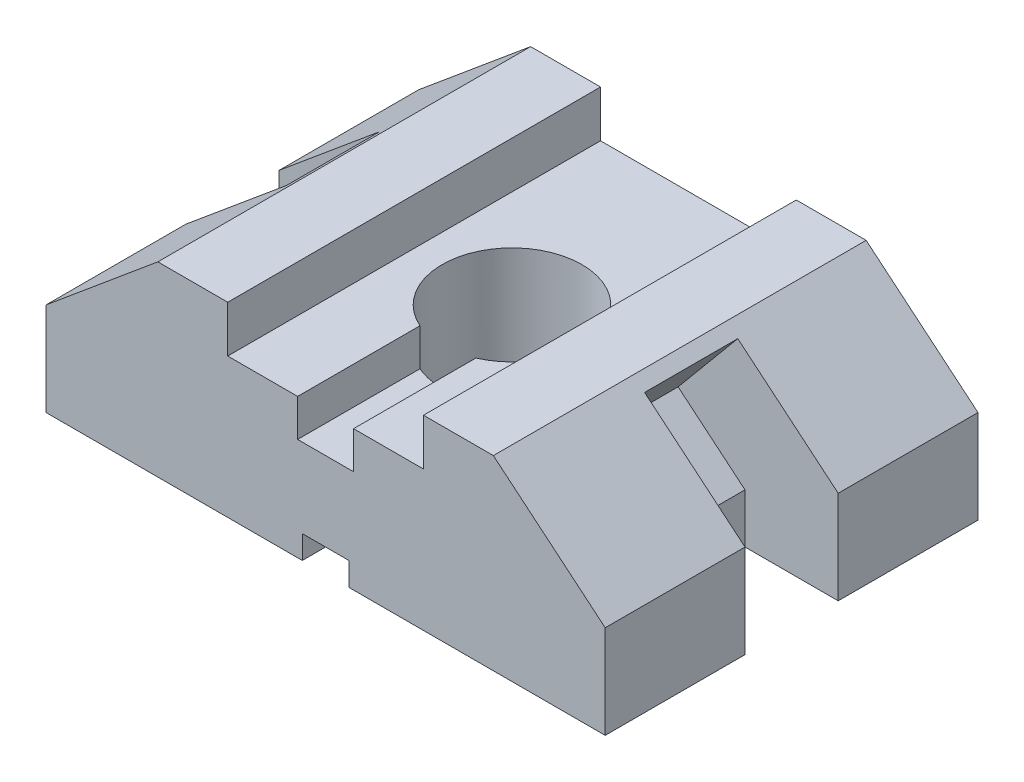
ISO-10303-21;
HEADER;
FILE_DESCRIPTION(('STEP AP214'),'2;1');
FILE_NAME('part.step','',(''),(''),'','','');
FILE_SCHEMA(('AUTOMOTIVE_DESIGN { 1 0 10303 214 1 1 1 1 }'));
ENDSEC;
DATA;
#1=APPLICATION_CONTEXT('core data for automotive mechanical design processes');
#2=APPLICATION_PROTOCOL_DEFINITION('international standard','automotive_design',2000,#1);
#3=PRODUCT_CONTEXT('',#1,'mechanical');
#4=PRODUCT('Part','Part','',(#3));
#5=PRODUCT_RELATED_PRODUCT_CATEGORY('part','',(#4));
#6=PRODUCT_DEFINITION_FORMATION('','',#4);
#7=PRODUCT_DEFINITION_CONTEXT('part definition',#1,'design');
#8=PRODUCT_DEFINITION('design','',#6,#7);
#9=PRODUCT_DEFINITION_SHAPE('','',#8);
#10=(LENGTH_UNIT() NAMED_UNIT(*) SI_UNIT(.MILLI.,.METRE.));
#11=(NAMED_UNIT(*) PLANE_ANGLE_UNIT() SI_UNIT($,.RADIAN.));
#12=(NAMED_UNIT(*) SI_UNIT($,.STERADIAN.) SOLID_ANGLE_UNIT());
#13=UNCERTAINTY_MEASURE_WITH_UNIT(LENGTH_MEASURE(1.E-05),#10,'distance_accuracy_value','');
#14=(GEOMETRIC_REPRESENTATION_CONTEXT(3) GLOBAL_UNCERTAINTY_ASSIGNED_CONTEXT((#13)) GLOBAL_UNIT_ASSIGNED_CONTEXT((#10,
#11,#12)) REPRESENTATION_CONTEXT('',''));
#15=CARTESIAN_POINT('',(0.,0.,0.));
#16=DIRECTION('',(0.,0.,1.));
#17=DIRECTION('',(1.,0.,0.));
#18=AXIS2_PLACEMENT_3D('',#15,#16,#17);
#19=CARTESIAN_POINT('',(0.,0.,80.));
#20=DIRECTION('',(1.,0.,0.));
#21=DIRECTION('',(0.,0.,-1.));
#22=AXIS2_PLACEMENT_3D('',#19,#20,#21);
#23=PLANE('',#22);
#24=DIRECTION('',(0.,0.,-1.));
#25=VECTOR('',#24,1.);
#26=CARTESIAN_POINT('',(0.,0.,80.));
#27=LINE('',#26,#25);
#28=CARTESIAN_POINT('',(0.,0.,30.));
#29=VERTEX_POINT('',#28);
#30=CARTESIAN_POINT('',(0.,0.,0.));
#31=VERTEX_POINT('',#30);
#32=EDGE_CURVE('E418',#29,#31,#27,.T.);
#33=ORIENTED_EDGE('',*,*,#32,.F.);
#34=DIRECTION('',(0.,-1.,0.));
#35=VECTOR('',#34,1.);
#36=CARTESIAN_POINT('',(0.,20.,30.));
#37=LINE('',#36,#35);
#38=CARTESIAN_POINT('',(0.,20.,30.));
#39=VERTEX_POINT('',#38);
#40=EDGE_CURVE('E286',#39,#29,#37,.T.);
#41=ORIENTED_EDGE('',*,*,#40,.F.);
#42=DIRECTION('',(0.,0.,-1.));
#43=VECTOR('',#42,1.);
#44=CARTESIAN_POINT('',(0.,20.,80.));
#45=LINE('',#44,#43);
#46=CARTESIAN_POINT('',(0.,20.,0.));
#47=VERTEX_POINT('',#46);
#48=EDGE_CURVE('E460',#39,#47,#45,.T.);
#49=ORIENTED_EDGE('',*,*,#48,.T.);
#50=DIRECTION('',(0.,-1.,0.));
#51=VECTOR('',#50,1.);
#52=CARTESIAN_POINT('',(0.,0.,0.));
#53=LINE('',#52,#51);
#54=EDGE_CURVE('E388',#47,#31,#53,.T.);
#55=ORIENTED_EDGE('',*,*,#54,.T.);
#56=EDGE_LOOP('',(#33,#41,#49,#55));
#57=FACE_BOUND('',#56,.T.);
#58=ADVANCED_FACE('F44',(#57),#23,.F.);
#59=CARTESIAN_POINT('',(120.,0.,80.));
#60=DIRECTION('',(-1.,0.,0.));
#61=DIRECTION('',(0.,0.,1.));
#62=AXIS2_PLACEMENT_3D('',#59,#60,#61);
#63=PLANE('',#62);
#64=DIRECTION('',(0.,0.,-1.));
#65=VECTOR('',#64,1.);
#66=CARTESIAN_POINT('',(120.,0.,80.));
#67=LINE('',#66,#65);
#68=CARTESIAN_POINT('',(120.,0.,80.));
#69=VERTEX_POINT('',#68);
#70=CARTESIAN_POINT('',(120.,0.,50.));
#71=VERTEX_POINT('',#70);
#72=EDGE_CURVE('E484',#69,#71,#67,.T.);
#73=ORIENTED_EDGE('',*,*,#72,.T.);
#74=DIRECTION('',(0.,-1.,0.));
#75=VECTOR('',#74,1.);
#76=CARTESIAN_POINT('',(120.,20.,50.));
#77=LINE('',#76,#75);
#78=CARTESIAN_POINT('',(120.,20.,50.));
#79=VERTEX_POINT('',#78);
#80=EDGE_CURVE('E321',#79,#71,#77,.T.);
#81=ORIENTED_EDGE('',*,*,#80,.F.);
#82=DIRECTION('',(0.,0.,-1.));
#83=VECTOR('',#82,1.);
#84=CARTESIAN_POINT('',(120.,20.,80.));
#85=LINE('',#84,#83);
#86=CARTESIAN_POINT('',(120.,20.,80.));
#87=VERTEX_POINT('',#86);
#88=EDGE_CURVE('E478',#87,#79,#85,.T.);
#89=ORIENTED_EDGE('',*,*,#88,.F.);
#90=DIRECTION('',(0.,1.,0.));
#91=VECTOR('',#90,1.);
#92=CARTESIAN_POINT('',(120.,0.,80.));
#93=LINE('',#92,#91);
#94=EDGE_CURVE('E398',#69,#87,#93,.T.);
#95=ORIENTED_EDGE('',*,*,#94,.F.);
#96=EDGE_LOOP('',(#73,#81,#89,#95));
#97=FACE_BOUND('',#96,.T.);
#98=ADVANCED_FACE('F549',(#97),#63,.F.);
#99=CARTESIAN_POINT('',(55.,0.,80.));
#100=DIRECTION('',(-1.,0.,0.));
#101=DIRECTION('',(0.,0.,1.));
#102=AXIS2_PLACEMENT_3D('',#99,#100,#101);
#103=PLANE('',#102);
#104=DIRECTION('',(0.,0.,-1.));
#105=VECTOR('',#104,1.);
#106=CARTESIAN_POINT('',(55.,0.,80.));
#107=LINE('',#106,#105);
#108=CARTESIAN_POINT('',(55.,0.,80.));
#109=VERTEX_POINT('',#108);
#110=CARTESIAN_POINT('',(55.,0.,54.142135623731));
#111=VERTEX_POINT('',#110);
#112=EDGE_CURVE('E499',#109,#111,#107,.T.);
#113=ORIENTED_EDGE('',*,*,#112,.T.);
#114=DIRECTION('',(0.,1.,0.));
#115=VECTOR('',#114,1.);
#116=CARTESIAN_POINT('',(55.,-50.,54.142135623731));
#117=LINE('',#116,#115);
#118=CARTESIAN_POINT('',(55.,5.,54.142135623731));
#119=VERTEX_POINT('',#118);
#120=EDGE_CURVE('E378',#111,#119,#117,.T.);
#121=ORIENTED_EDGE('',*,*,#120,.T.);
#122=DIRECTION('',(0.,0.,-1.));
#123=VECTOR('',#122,1.);
#124=CARTESIAN_POINT('',(55.,5.,80.));
#125=LINE('',#124,#123);
#126=CARTESIAN_POINT('',(55.,5.,80.));
#127=VERTEX_POINT('',#126);
#128=EDGE_CURVE('E496',#127,#119,#125,.T.);
#129=ORIENTED_EDGE('',*,*,#128,.F.);
#130=DIRECTION('',(0.,1.,0.));
#131=VECTOR('',#130,1.);
#132=CARTESIAN_POINT('',(55.,0.,80.));
#133=LINE('',#132,#131);
#134=EDGE_CURVE('E386',#109,#127,#133,.T.);
#135=ORIENTED_EDGE('',*,*,#134,.F.);
#136=EDGE_LOOP('',(#113,#121,#129,#135));
#137=FACE_BOUND('',#136,.T.);
#138=ADVANCED_FACE('F568',(#137),#103,.F.);
#139=CARTESIAN_POINT('',(55.,5.,80.));
#140=DIRECTION('',(0.,1.,0.));
#141=DIRECTION('',(0.,0.,1.));
#142=AXIS2_PLACEMENT_3D('',#139,#140,#141);
#143=PLANE('',#142);
#144=DIRECTION('',(0.,0.,-1.));
#145=VECTOR('',#144,1.);
#146=CARTESIAN_POINT('',(65.,5.,80.));
#147=LINE('',#146,#145);
#148=CARTESIAN_POINT('',(65.,5.,25.857864376269));
#149=VERTEX_POINT('',#148);
#150=CARTESIAN_POINT('',(65.,5.,0.));
#151=VERTEX_POINT('',#150);
#152=EDGE_CURVE('E493',#149,#151,#147,.T.);
#153=ORIENTED_EDGE('',*,*,#152,.F.);
#154=CARTESIAN_POINT('',(60.,5.,40.));
#155=DIRECTION('',(0.,1.,0.));
#156=DIRECTION('',(0.,0.,1.));
#157=AXIS2_PLACEMENT_3D('',#154,#155,#156);
#158=CIRCLE('',#157,15.);
#159=CARTESIAN_POINT('',(55.,5.,25.8578643762691));
#160=VERTEX_POINT('',#159);
#161=EDGE_CURVE('E374',#149,#160,#158,.T.);
#162=ORIENTED_EDGE('',*,*,#161,.T.);
#163=CARTESIAN_POINT('',(55.,5.,0.));
#164=VERTEX_POINT('',#163);
#165=EDGE_CURVE('E492',#160,#164,#125,.T.);
#166=ORIENTED_EDGE('',*,*,#165,.T.);
#167=DIRECTION('',(1.,0.,0.));
#168=VECTOR('',#167,1.);
#169=CARTESIAN_POINT('',(55.,5.,0.));
#170=LINE('',#169,#168);
#171=EDGE_CURVE('E425',#164,#151,#170,.T.);
#172=ORIENTED_EDGE('',*,*,#171,.T.);
#173=EDGE_LOOP('',(#153,#162,#166,#172));
#174=FACE_BOUND('',#173,.T.);
#175=ADVANCED_FACE('F590',(#174),#143,.F.);
#176=CARTESIAN_POINT('',(65.,5.,80.));
#177=DIRECTION('',(1.,0.,0.));
#178=DIRECTION('',(0.,0.,-1.));
#179=AXIS2_PLACEMENT_3D('',#176,#177,#178);
#180=PLANE('',#179);
#181=DIRECTION('',(0.,0.,-1.));
#182=VECTOR('',#181,1.);
#183=CARTESIAN_POINT('',(65.,0.,80.));
#184=LINE('',#183,#182);
#185=CARTESIAN_POINT('',(65.,0.,25.857864376269));
#186=VERTEX_POINT('',#185);
#187=CARTESIAN_POINT('',(65.,0.,0.));
#188=VERTEX_POINT('',#187);
#189=EDGE_CURVE('E487',#186,#188,#184,.T.);
#190=ORIENTED_EDGE('',*,*,#189,.F.);
#191=DIRECTION('',(0.,1.,0.));
#192=VECTOR('',#191,1.);
#193=CARTESIAN_POINT('',(65.,-50.,25.857864376269));
#194=LINE('',#193,#192);
#195=EDGE_CURVE('E367',#186,#149,#194,.T.);
#196=ORIENTED_EDGE('',*,*,#195,.T.);
#197=ORIENTED_EDGE('',*,*,#152,.T.);
#198=DIRECTION('',(0.,-1.,0.));
#199=VECTOR('',#198,1.);
#200=CARTESIAN_POINT('',(65.,5.,0.));
#201=LINE('',#200,#199);
#202=EDGE_CURVE('E430',#151,#188,#201,.T.);
#203=ORIENTED_EDGE('',*,*,#202,.T.);
#204=EDGE_LOOP('',(#190,#196,#197,#203));
#205=FACE_BOUND('',#204,.T.);
#206=ADVANCED_FACE('F588',(#205),#180,.F.);
#207=CARTESIAN_POINT('',(0.,0.,80.));
#208=DIRECTION('',(0.,1.,0.));
#209=DIRECTION('',(0.,0.,1.));
#210=AXIS2_PLACEMENT_3D('',#207,#208,#209);
#211=PLANE('',#210);
#212=DIRECTION('',(0.,0.,1.));
#213=VECTOR('',#212,1.);
#214=CARTESIAN_POINT('',(20.,0.,30.));
#215=LINE('',#214,#213);
#216=CARTESIAN_POINT('',(20.,0.,30.));
#217=VERTEX_POINT('',#216);
#218=CARTESIAN_POINT('',(20.,0.,50.));
#219=VERTEX_POINT('',#218);
#220=EDGE_CURVE('E295',#217,#219,#215,.T.);
#221=ORIENTED_EDGE('',*,*,#220,.F.);
#222=DIRECTION('',(-1.,0.,0.));
#223=VECTOR('',#222,1.);
#224=CARTESIAN_POINT('',(20.,0.,30.));
#225=LINE('',#224,#223);
#226=EDGE_CURVE('E297',#217,#29,#225,.T.);
#227=ORIENTED_EDGE('',*,*,#226,.T.);
#228=ORIENTED_EDGE('',*,*,#32,.T.);
#229=DIRECTION('',(1.,0.,0.));
#230=VECTOR('',#229,1.);
#231=CARTESIAN_POINT('',(0.,0.,0.));
#232=LINE('',#231,#230);
#233=CARTESIAN_POINT('',(55.,0.,0.));
#234=VERTEX_POINT('',#233);
#235=EDGE_CURVE('E383',#31,#234,#232,.T.);
#236=ORIENTED_EDGE('',*,*,#235,.T.);
#237=CARTESIAN_POINT('',(55.,0.,25.8578643762691));
#238=VERTEX_POINT('',#237);
#239=EDGE_CURVE('E497',#238,#234,#107,.T.);
#240=ORIENTED_EDGE('',*,*,#239,.F.);
#241=CARTESIAN_POINT('',(60.,0.,40.));
#242=DIRECTION('',(0.,1.,0.));
#243=DIRECTION('',(0.,0.,1.));
#244=AXIS2_PLACEMENT_3D('',#241,#242,#243);
#245=CIRCLE('',#244,15.);
#246=EDGE_CURVE('E385',#238,#111,#245,.T.);
#247=ORIENTED_EDGE('',*,*,#246,.T.);
#248=ORIENTED_EDGE('',*,*,#112,.F.);
#249=DIRECTION('',(1.,0.,0.));
#250=VECTOR('',#249,1.);
#251=CARTESIAN_POINT('',(0.,0.,80.));
#252=LINE('',#251,#250);
#253=CARTESIAN_POINT('',(0.,0.,80.));
#254=VERTEX_POINT('',#253);
#255=EDGE_CURVE('E387',#254,#109,#252,.T.);
#256=ORIENTED_EDGE('',*,*,#255,.F.);
#257=CARTESIAN_POINT('',(0.,0.,50.));
#258=VERTEX_POINT('',#257);
#259=EDGE_CURVE('E451',#254,#258,#27,.T.);
#260=ORIENTED_EDGE('',*,*,#259,.T.);
#261=DIRECTION('',(-1.,0.,0.));
#262=VECTOR('',#261,1.);
#263=CARTESIAN_POINT('',(20.,0.,50.));
#264=LINE('',#263,#262);
#265=EDGE_CURVE('E70',#219,#258,#264,.T.);
#266=ORIENTED_EDGE('',*,*,#265,.F.);
#267=EDGE_LOOP('',(#221,#227,#228,#236,#240,#247,#248,#256,#260,#266));
#268=FACE_BOUND('',#267,.T.);
#269=ADVANCED_FACE('F50',(#268),#211,.F.);
#270=ORIENTED_EDGE('',*,*,#165,.F.);
#271=DIRECTION('',(0.,1.,0.));
#272=VECTOR('',#271,1.);
#273=CARTESIAN_POINT('',(55.,-50.,25.8578643762691));
#274=LINE('',#273,#272);
#275=EDGE_CURVE('E376',#160,#238,#274,.F.);
#276=ORIENTED_EDGE('',*,*,#275,.T.);
#277=ORIENTED_EDGE('',*,*,#239,.T.);
#278=DIRECTION('',(0.,1.,0.));
#279=VECTOR('',#278,1.);
#280=CARTESIAN_POINT('',(55.,0.,0.));
#281=LINE('',#280,#279);
#282=EDGE_CURVE('E423',#234,#164,#281,.T.);
#283=ORIENTED_EDGE('',*,*,#282,.T.);
#284=EDGE_LOOP('',(#270,#276,#277,#283));
#285=FACE_BOUND('',#284,.T.);
#286=ADVANCED_FACE('F579',(#285),#103,.F.);
#287=ORIENTED_EDGE('',*,*,#128,.T.);
#288=CARTESIAN_POINT('',(65.,5.,54.142135623731));
#289=VERTEX_POINT('',#288);
#290=EDGE_CURVE('E375',#119,#289,#158,.T.);
#291=ORIENTED_EDGE('',*,*,#290,.T.);
#292=CARTESIAN_POINT('',(65.,5.,80.));
#293=VERTEX_POINT('',#292);
#294=EDGE_CURVE('E495',#293,#289,#147,.T.);
#295=ORIENTED_EDGE('',*,*,#294,.F.);
#296=DIRECTION('',(1.,0.,0.));
#297=VECTOR('',#296,1.);
#298=CARTESIAN_POINT('',(55.,5.,80.));
#299=LINE('',#298,#297);
#300=EDGE_CURVE('E395',#127,#293,#299,.T.);
#301=ORIENTED_EDGE('',*,*,#300,.F.);
#302=EDGE_LOOP('',(#287,#291,#295,#301));
#303=FACE_BOUND('',#302,.T.);
#304=ADVANCED_FACE('F562',(#303),#143,.F.);
#305=ORIENTED_EDGE('',*,*,#294,.T.);
#306=DIRECTION('',(0.,1.,0.));
#307=VECTOR('',#306,1.);
#308=CARTESIAN_POINT('',(65.,-50.,54.142135623731));
#309=LINE('',#308,#307);
#310=CARTESIAN_POINT('',(65.,0.,54.142135623731));
#311=VERTEX_POINT('',#310);
#312=EDGE_CURVE('E366',#289,#311,#309,.F.);
#313=ORIENTED_EDGE('',*,*,#312,.T.);
#314=CARTESIAN_POINT('',(65.,0.,80.));
#315=VERTEX_POINT('',#314);
#316=EDGE_CURVE('E486',#315,#311,#184,.T.);
#317=ORIENTED_EDGE('',*,*,#316,.F.);
#318=DIRECTION('',(0.,-1.,0.));
#319=VECTOR('',#318,1.);
#320=CARTESIAN_POINT('',(65.,5.,80.));
#321=LINE('',#320,#319);
#322=EDGE_CURVE('E391',#293,#315,#321,.T.);
#323=ORIENTED_EDGE('',*,*,#322,.F.);
#324=EDGE_LOOP('',(#305,#313,#317,#323));
#325=FACE_BOUND('',#324,.T.);
#326=ADVANCED_FACE('F559',(#325),#180,.F.);
#327=CARTESIAN_POINT('',(65.,0.,80.));
#328=DIRECTION('',(0.,1.,0.));
#329=DIRECTION('',(0.,0.,1.));
#330=AXIS2_PLACEMENT_3D('',#327,#328,#329);
#331=PLANE('',#330);
#332=DIRECTION('',(0.,0.,-1.));
#333=VECTOR('',#332,1.);
#334=CARTESIAN_POINT('',(100.,0.,50.));
#335=LINE('',#334,#333);
#336=CARTESIAN_POINT('',(100.,0.,50.));
#337=VERTEX_POINT('',#336);
#338=CARTESIAN_POINT('',(100.,0.,30.));
#339=VERTEX_POINT('',#338);
#340=EDGE_CURVE('E329',#337,#339,#335,.T.);
#341=ORIENTED_EDGE('',*,*,#340,.F.);
#342=DIRECTION('',(1.,0.,0.));
#343=VECTOR('',#342,1.);
#344=CARTESIAN_POINT('',(100.,0.,50.));
#345=LINE('',#344,#343);
#346=EDGE_CURVE('E331',#337,#71,#345,.T.);
#347=ORIENTED_EDGE('',*,*,#346,.T.);
#348=ORIENTED_EDGE('',*,*,#72,.F.);
#349=DIRECTION('',(1.,0.,0.));
#350=VECTOR('',#349,1.);
#351=CARTESIAN_POINT('',(65.,0.,80.));
#352=LINE('',#351,#350);
#353=EDGE_CURVE('E397',#315,#69,#352,.T.);
#354=ORIENTED_EDGE('',*,*,#353,.F.);
#355=ORIENTED_EDGE('',*,*,#316,.T.);
#356=CARTESIAN_POINT('',(60.,0.,40.));
#357=DIRECTION('',(0.,1.,0.));
#358=DIRECTION('',(0.,0.,1.));
#359=AXIS2_PLACEMENT_3D('',#356,#357,#358);
#360=CIRCLE('',#359,15.);
#361=EDGE_CURVE('E361',#311,#186,#360,.T.);
#362=ORIENTED_EDGE('',*,*,#361,.T.);
#363=ORIENTED_EDGE('',*,*,#189,.T.);
#364=DIRECTION('',(1.,0.,0.));
#365=VECTOR('',#364,1.);
#366=CARTESIAN_POINT('',(65.,0.,0.));
#367=LINE('',#366,#365);
#368=CARTESIAN_POINT('',(120.,0.,0.));
#369=VERTEX_POINT('',#368);
#370=EDGE_CURVE('E427',#188,#369,#367,.T.);
#371=ORIENTED_EDGE('',*,*,#370,.T.);
#372=CARTESIAN_POINT('',(120.,0.,30.));
#373=VERTEX_POINT('',#372);
#374=EDGE_CURVE('E483',#373,#369,#67,.T.);
#375=ORIENTED_EDGE('',*,*,#374,.F.);
#376=DIRECTION('',(1.,0.,0.));
#377=VECTOR('',#376,1.);
#378=CARTESIAN_POINT('',(100.,0.,30.));
#379=LINE('',#378,#377);
#380=EDGE_CURVE('E339',#339,#373,#379,.T.);
#381=ORIENTED_EDGE('',*,*,#380,.F.);
#382=EDGE_LOOP('',(#341,#347,#348,#354,#355,#362,#363,#371,#375,#381));
#383=FACE_BOUND('',#382,.T.);
#384=ADVANCED_FACE('F528',(#383),#331,.F.);
#385=CARTESIAN_POINT('',(120.,20.,30.));
#386=VERTEX_POINT('',#385);
#387=CARTESIAN_POINT('',(120.,20.,0.));
#388=VERTEX_POINT('',#387);
#389=EDGE_CURVE('E476',#386,#388,#85,.T.);
#390=ORIENTED_EDGE('',*,*,#389,.F.);
#391=DIRECTION('',(0.,1.,0.));
#392=VECTOR('',#391,1.);
#393=CARTESIAN_POINT('',(120.,20.,30.));
#394=LINE('',#393,#392);
#395=EDGE_CURVE('E326',#373,#386,#394,.T.);
#396=ORIENTED_EDGE('',*,*,#395,.F.);
#397=ORIENTED_EDGE('',*,*,#374,.T.);
#398=DIRECTION('',(0.,1.,0.));
#399=VECTOR('',#398,1.);
#400=CARTESIAN_POINT('',(120.,0.,0.));
#401=LINE('',#400,#399);
#402=EDGE_CURVE('E433',#369,#388,#401,.T.);
#403=ORIENTED_EDGE('',*,*,#402,.T.);
#404=EDGE_LOOP('',(#390,#396,#397,#403));
#405=FACE_BOUND('',#404,.T.);
#406=ADVANCED_FACE('F535',(#405),#63,.F.);
#407=CARTESIAN_POINT('',(96.,40.,80.));
#408=DIRECTION('',(-0.64018439966448,-0.768221279597376,0.));
#409=DIRECTION('',(0.768221279597376,-0.64018439966448,0.));
#410=AXIS2_PLACEMENT_3D('',#407,#408,#409);
#411=PLANE('',#410);
#412=DIRECTION('',(0.,0.,1.));
#413=VECTOR('',#412,1.);
#414=CARTESIAN_POINT('',(98.4512258008987,37.9573118325844,50.));
#415=LINE('',#414,#413);
#416=CARTESIAN_POINT('',(98.4512258008987,37.9573118325844,30.));
#417=VERTEX_POINT('',#416);
#418=CARTESIAN_POINT('',(98.4512258008987,37.9573118325844,50.));
#419=VERTEX_POINT('',#418);
#420=EDGE_CURVE('E319',#417,#419,#415,.T.);
#421=ORIENTED_EDGE('',*,*,#420,.F.);
#422=DIRECTION('',(-0.768221279597376,0.64018439966448,0.));
#423=VECTOR('',#422,1.);
#424=CARTESIAN_POINT('',(98.4512258008987,37.9573118325844,30.));
#425=LINE('',#424,#423);
#426=EDGE_CURVE('E302',#386,#417,#425,.T.);
#427=ORIENTED_EDGE('',*,*,#426,.F.);
#428=ORIENTED_EDGE('',*,*,#389,.T.);
#429=DIRECTION('',(-0.768221279597376,0.64018439966448,0.));
#430=VECTOR('',#429,1.);
#431=CARTESIAN_POINT('',(96.,40.,0.));
#432=LINE('',#431,#430);
#433=CARTESIAN_POINT('',(96.,40.,0.));
#434=VERTEX_POINT('',#433);
#435=EDGE_CURVE('E436',#388,#434,#432,.T.);
#436=ORIENTED_EDGE('',*,*,#435,.T.);
#437=DIRECTION('',(0.,0.,-1.));
#438=VECTOR('',#437,1.);
#439=CARTESIAN_POINT('',(96.,40.,80.));
#440=LINE('',#439,#438);
#441=CARTESIAN_POINT('',(96.,40.,80.));
#442=VERTEX_POINT('',#441);
#443=EDGE_CURVE('E477',#442,#434,#440,.T.);
#444=ORIENTED_EDGE('',*,*,#443,.F.);
#445=DIRECTION('',(-0.768221279597376,0.64018439966448,0.));
#446=VECTOR('',#445,1.);
#447=CARTESIAN_POINT('',(96.,40.,80.));
#448=LINE('',#447,#446);
#449=EDGE_CURVE('E396',#87,#442,#448,.T.);
#450=ORIENTED_EDGE('',*,*,#449,.F.);
#451=ORIENTED_EDGE('',*,*,#88,.T.);
#452=DIRECTION('',(0.768221279597376,-0.64018439966448,0.));
#453=VECTOR('',#452,1.);
#454=CARTESIAN_POINT('',(120.,20.,50.));
#455=LINE('',#454,#453);
#456=EDGE_CURVE('E309',#419,#79,#455,.T.);
#457=ORIENTED_EDGE('',*,*,#456,.F.);
#458=EDGE_LOOP('',(#421,#427,#428,#436,#444,#450,#451,#457));
#459=FACE_BOUND('',#458,.T.);
#460=ADVANCED_FACE('F540',(#459),#411,.F.);
#461=CARTESIAN_POINT('',(81.,40.,80.));
#462=DIRECTION('',(0.,-1.,0.));
#463=DIRECTION('',(0.,0.,-1.));
#464=AXIS2_PLACEMENT_3D('',#461,#462,#463);
#465=PLANE('',#464);
#466=DIRECTION('',(-1.,0.,0.));
#467=VECTOR('',#466,1.);
#468=CARTESIAN_POINT('',(81.,40.,0.));
#469=LINE('',#468,#467);
#470=CARTESIAN_POINT('',(81.,40.,0.));
#471=VERTEX_POINT('',#470);
#472=EDGE_CURVE('E438',#434,#471,#469,.T.);
#473=ORIENTED_EDGE('',*,*,#472,.T.);
#474=DIRECTION('',(0.,0.,-1.));
#475=VECTOR('',#474,1.);
#476=CARTESIAN_POINT('',(81.,40.,80.));
#477=LINE('',#476,#475);
#478=CARTESIAN_POINT('',(81.,40.,80.));
#479=VERTEX_POINT('',#478);
#480=EDGE_CURVE('E474',#479,#471,#477,.T.);
#481=ORIENTED_EDGE('',*,*,#480,.F.);
#482=DIRECTION('',(-1.,0.,0.));
#483=VECTOR('',#482,1.);
#484=CARTESIAN_POINT('',(81.,40.,80.));
#485=LINE('',#484,#483);
#486=EDGE_CURVE('E405',#442,#479,#485,.T.);
#487=ORIENTED_EDGE('',*,*,#486,.F.);
#488=ORIENTED_EDGE('',*,*,#443,.T.);
#489=EDGE_LOOP('',(#473,#481,#487,#488));
#490=FACE_BOUND('',#489,.T.);
#491=ADVANCED_FACE('F591',(#490),#465,.F.);
#492=CARTESIAN_POINT('',(81.,30.,80.));
#493=DIRECTION('',(1.,0.,0.));
#494=DIRECTION('',(0.,0.,-1.));
#495=AXIS2_PLACEMENT_3D('',#492,#493,#494);
#496=PLANE('',#495);
#497=DIRECTION('',(0.,-1.,0.));
#498=VECTOR('',#497,1.);
#499=CARTESIAN_POINT('',(81.,30.,0.));
#500=LINE('',#499,#498);
#501=CARTESIAN_POINT('',(81.,30.,0.));
#502=VERTEX_POINT('',#501);
#503=EDGE_CURVE('E439',#471,#502,#500,.T.);
#504=ORIENTED_EDGE('',*,*,#503,.T.);
#505=DIRECTION('',(0.,0.,-1.));
#506=VECTOR('',#505,1.);
#507=CARTESIAN_POINT('',(81.,30.,80.));
#508=LINE('',#507,#506);
#509=CARTESIAN_POINT('',(81.,30.,80.));
#510=VERTEX_POINT('',#509);
#511=EDGE_CURVE('E468',#510,#502,#508,.T.);
#512=ORIENTED_EDGE('',*,*,#511,.F.);
#513=DIRECTION('',(0.,-1.,0.));
#514=VECTOR('',#513,1.);
#515=CARTESIAN_POINT('',(81.,30.,80.));
#516=LINE('',#515,#514);
#517=EDGE_CURVE('E404',#479,#510,#516,.T.);
#518=ORIENTED_EDGE('',*,*,#517,.F.);
#519=ORIENTED_EDGE('',*,*,#480,.T.);
#520=EDGE_LOOP('',(#504,#512,#518,#519));
#521=FACE_BOUND('',#520,.T.);
#522=ADVANCED_FACE('F599',(#521),#496,.F.);
#523=CARTESIAN_POINT('',(54.,30.,80.));
#524=DIRECTION('',(0.,-1.,0.));
#525=DIRECTION('',(0.,0.,-1.));
#526=AXIS2_PLACEMENT_3D('',#523,#524,#525);
#527=PLANE('',#526);
#528=CARTESIAN_POINT('',(60.,30.,40.));
#529=DIRECTION('',(0.,1.,0.));
#530=DIRECTION('',(0.,0.,1.));
#531=AXIS2_PLACEMENT_3D('',#528,#529,#530);
#532=CIRCLE('',#531,15.);
#533=CARTESIAN_POINT('',(66.,30.,53.7477270848675));
#534=VERTEX_POINT('',#533);
#535=CARTESIAN_POINT('',(54.,30.,53.7477270848675));
#536=VERTEX_POINT('',#535);
#537=EDGE_CURVE('E351',#534,#536,#532,.T.);
#538=ORIENTED_EDGE('',*,*,#537,.F.);
#539=DIRECTION('',(0.,0.,1.));
#540=VECTOR('',#539,1.);
#541=CARTESIAN_POINT('',(66.,30.,50.));
#542=LINE('',#541,#540);
#543=CARTESIAN_POINT('',(66.,30.,80.));
#544=VERTEX_POINT('',#543);
#545=EDGE_CURVE('E355',#534,#544,#542,.T.);
#546=ORIENTED_EDGE('',*,*,#545,.T.);
#547=DIRECTION('',(-1.,0.,0.));
#548=VECTOR('',#547,1.);
#549=CARTESIAN_POINT('',(66.,30.,80.));
#550=LINE('',#549,#548);
#551=EDGE_CURVE('E410',#510,#544,#550,.T.);
#552=ORIENTED_EDGE('',*,*,#551,.F.);
#553=ORIENTED_EDGE('',*,*,#511,.T.);
#554=DIRECTION('',(-1.,0.,0.));
#555=VECTOR('',#554,1.);
#556=CARTESIAN_POINT('',(54.,30.,0.));
#557=LINE('',#556,#555);
#558=CARTESIAN_POINT('',(39.,30.,0.));
#559=VERTEX_POINT('',#558);
#560=EDGE_CURVE('E442',#502,#559,#557,.T.);
#561=ORIENTED_EDGE('',*,*,#560,.T.);
#562=DIRECTION('',(0.,0.,-1.));
#563=VECTOR('',#562,1.);
#564=CARTESIAN_POINT('',(39.,30.,80.));
#565=LINE('',#564,#563);
#566=CARTESIAN_POINT('',(39.,30.,80.));
#567=VERTEX_POINT('',#566);
#568=EDGE_CURVE('E470',#567,#559,#565,.T.);
#569=ORIENTED_EDGE('',*,*,#568,.F.);
#570=CARTESIAN_POINT('',(54.,30.,80.));
#571=VERTEX_POINT('',#570);
#572=EDGE_CURVE('E407',#571,#567,#550,.T.);
#573=ORIENTED_EDGE('',*,*,#572,.F.);
#574=DIRECTION('',(0.,0.,1.));
#575=VECTOR('',#574,1.);
#576=CARTESIAN_POINT('',(54.,30.,50.));
#577=LINE('',#576,#575);
#578=EDGE_CURVE('E352',#536,#571,#577,.T.);
#579=ORIENTED_EDGE('',*,*,#578,.F.);
#580=EDGE_LOOP('',(#538,#546,#552,#553,#561,#569,#573,#579));
#581=FACE_BOUND('',#580,.T.);
#582=ADVANCED_FACE('F603',(#581),#527,.F.);
#583=CARTESIAN_POINT('',(39.,30.,80.));
#584=DIRECTION('',(-1.,0.,0.));
#585=DIRECTION('',(0.,0.,1.));
#586=AXIS2_PLACEMENT_3D('',#583,#584,#585);
#587=PLANE('',#586);
#588=DIRECTION('',(0.,1.,0.));
#589=VECTOR('',#588,1.);
#590=CARTESIAN_POINT('',(39.,30.,0.));
#591=LINE('',#590,#589);
#592=CARTESIAN_POINT('',(39.,40.,0.));
#593=VERTEX_POINT('',#592);
#594=EDGE_CURVE('E444',#559,#593,#591,.T.);
#595=ORIENTED_EDGE('',*,*,#594,.T.);
#596=DIRECTION('',(0.,0.,-1.));
#597=VECTOR('',#596,1.);
#598=CARTESIAN_POINT('',(39.,40.,80.));
#599=LINE('',#598,#597);
#600=CARTESIAN_POINT('',(39.,40.,80.));
#601=VERTEX_POINT('',#600);
#602=EDGE_CURVE('E464',#601,#593,#599,.T.);
#603=ORIENTED_EDGE('',*,*,#602,.F.);
#604=DIRECTION('',(0.,1.,0.));
#605=VECTOR('',#604,1.);
#606=CARTESIAN_POINT('',(39.,30.,80.));
#607=LINE('',#606,#605);
#608=EDGE_CURVE('E408',#567,#601,#607,.T.);
#609=ORIENTED_EDGE('',*,*,#608,.F.);
#610=ORIENTED_EDGE('',*,*,#568,.T.);
#611=EDGE_LOOP('',(#595,#603,#609,#610));
#612=FACE_BOUND('',#611,.T.);
#613=ADVANCED_FACE('F625',(#612),#587,.F.);
#614=CARTESIAN_POINT('',(39.,40.,80.));
#615=DIRECTION('',(0.,-1.,0.));
#616=DIRECTION('',(0.,0.,-1.));
#617=AXIS2_PLACEMENT_3D('',#614,#615,#616);
#618=PLANE('',#617);
#619=DIRECTION('',(-1.,0.,0.));
#620=VECTOR('',#619,1.);
#621=CARTESIAN_POINT('',(39.,40.,0.));
#622=LINE('',#621,#620);
#623=CARTESIAN_POINT('',(24.,40.,0.));
#624=VERTEX_POINT('',#623);
#625=EDGE_CURVE('E450',#593,#624,#622,.T.);
#626=ORIENTED_EDGE('',*,*,#625,.T.);
#627=DIRECTION('',(0.,0.,-1.));
#628=VECTOR('',#627,1.);
#629=CARTESIAN_POINT('',(24.,40.,80.));
#630=LINE('',#629,#628);
#631=CARTESIAN_POINT('',(24.,40.,80.));
#632=VERTEX_POINT('',#631);
#633=EDGE_CURVE('E462',#632,#624,#630,.T.);
#634=ORIENTED_EDGE('',*,*,#633,.F.);
#635=DIRECTION('',(-1.,0.,0.));
#636=VECTOR('',#635,1.);
#637=CARTESIAN_POINT('',(39.,40.,80.));
#638=LINE('',#637,#636);
#639=EDGE_CURVE('E415',#601,#632,#638,.T.);
#640=ORIENTED_EDGE('',*,*,#639,.F.);
#641=ORIENTED_EDGE('',*,*,#602,.T.);
#642=EDGE_LOOP('',(#626,#634,#640,#641));
#643=FACE_BOUND('',#642,.T.);
#644=ADVANCED_FACE('F628',(#643),#618,.F.);
#645=CARTESIAN_POINT('',(24.,40.,80.));
#646=DIRECTION('',(0.64018439966448,-0.768221279597376,0.));
#647=DIRECTION('',(0.768221279597376,0.64018439966448,0.));
#648=AXIS2_PLACEMENT_3D('',#645,#646,#647);
#649=PLANE('',#648);
#650=ORIENTED_EDGE('',*,*,#48,.F.);
#651=DIRECTION('',(-0.768221279597376,-0.64018439966448,0.));
#652=VECTOR('',#651,1.);
#653=CARTESIAN_POINT('',(0.,20.,30.));
#654=LINE('',#653,#652);
#655=CARTESIAN_POINT('',(21.6499498332045,38.0416248610038,30.));
#656=VERTEX_POINT('',#655);
#657=EDGE_CURVE('E272',#656,#39,#654,.T.);
#658=ORIENTED_EDGE('',*,*,#657,.F.);
#659=DIRECTION('',(0.,0.,-1.));
#660=VECTOR('',#659,1.);
#661=CARTESIAN_POINT('',(21.6499498332045,38.0416248610038,30.));
#662=LINE('',#661,#660);
#663=CARTESIAN_POINT('',(21.6499498332045,38.0416248610038,50.));
#664=VERTEX_POINT('',#663);
#665=EDGE_CURVE('E290',#664,#656,#662,.T.);
#666=ORIENTED_EDGE('',*,*,#665,.F.);
#667=DIRECTION('',(0.768221279597376,0.64018439966448,0.));
#668=VECTOR('',#667,1.);
#669=CARTESIAN_POINT('',(21.6499498332045,38.0416248610038,50.));
#670=LINE('',#669,#668);
#671=CARTESIAN_POINT('',(0.,20.,50.));
#672=VERTEX_POINT('',#671);
#673=EDGE_CURVE('E277',#672,#664,#670,.T.);
#674=ORIENTED_EDGE('',*,*,#673,.F.);
#675=CARTESIAN_POINT('',(0.,20.,80.));
#676=VERTEX_POINT('',#675);
#677=EDGE_CURVE('E459',#676,#672,#45,.T.);
#678=ORIENTED_EDGE('',*,*,#677,.F.);
#679=DIRECTION('',(-0.768221279597376,-0.64018439966448,0.));
#680=VECTOR('',#679,1.);
#681=CARTESIAN_POINT('',(24.,40.,80.));
#682=LINE('',#681,#680);
#683=EDGE_CURVE('E411',#632,#676,#682,.T.);
#684=ORIENTED_EDGE('',*,*,#683,.F.);
#685=ORIENTED_EDGE('',*,*,#633,.T.);
#686=DIRECTION('',(-0.768221279597376,-0.64018439966448,0.));
#687=VECTOR('',#686,1.);
#688=CARTESIAN_POINT('',(24.,40.,0.));
#689=LINE('',#688,#687);
#690=EDGE_CURVE('E446',#624,#47,#689,.T.);
#691=ORIENTED_EDGE('',*,*,#690,.T.);
#692=EDGE_LOOP('',(#650,#658,#666,#674,#678,#684,#685,#691));
#693=FACE_BOUND('',#692,.T.);
#694=ADVANCED_FACE('F633',(#693),#649,.F.);
#695=ORIENTED_EDGE('',*,*,#677,.T.);
#696=DIRECTION('',(0.,1.,0.));
#697=VECTOR('',#696,1.);
#698=CARTESIAN_POINT('',(0.,20.,50.));
#699=LINE('',#698,#697);
#700=EDGE_CURVE('E294',#258,#672,#699,.T.);
#701=ORIENTED_EDGE('',*,*,#700,.F.);
#702=ORIENTED_EDGE('',*,*,#259,.F.);
#703=DIRECTION('',(0.,-1.,0.));
#704=VECTOR('',#703,1.);
#705=CARTESIAN_POINT('',(0.,0.,80.));
#706=LINE('',#705,#704);
#707=EDGE_CURVE('E417',#676,#254,#706,.T.);
#708=ORIENTED_EDGE('',*,*,#707,.F.);
#709=EDGE_LOOP('',(#695,#701,#702,#708));
#710=FACE_BOUND('',#709,.T.);
#711=ADVANCED_FACE('F640',(#710),#23,.F.);
#712=CARTESIAN_POINT('',(0.,0.,80.));
#713=DIRECTION('',(0.,0.,1.));
#714=DIRECTION('',(1.,0.,0.));
#715=AXIS2_PLACEMENT_3D('',#712,#713,#714);
#716=PLANE('',#715);
#717=DIRECTION('',(0.,1.,0.));
#718=VECTOR('',#717,1.);
#719=CARTESIAN_POINT('',(66.,22.,80.));
#720=LINE('',#719,#718);
#721=CARTESIAN_POINT('',(66.,22.,80.));
#722=VERTEX_POINT('',#721);
#723=EDGE_CURVE('E346',#722,#544,#720,.T.);
#724=ORIENTED_EDGE('',*,*,#723,.F.);
#725=DIRECTION('',(1.,0.,0.));
#726=VECTOR('',#725,1.);
#727=CARTESIAN_POINT('',(54.,22.,80.));
#728=LINE('',#727,#726);
#729=CARTESIAN_POINT('',(54.,22.,80.));
#730=VERTEX_POINT('',#729);
#731=EDGE_CURVE('E347',#730,#722,#728,.T.);
#732=ORIENTED_EDGE('',*,*,#731,.F.);
#733=DIRECTION('',(0.,-1.,0.));
#734=VECTOR('',#733,1.);
#735=CARTESIAN_POINT('',(54.,30.,80.));
#736=LINE('',#735,#734);
#737=EDGE_CURVE('E342',#571,#730,#736,.T.);
#738=ORIENTED_EDGE('',*,*,#737,.F.);
#739=ORIENTED_EDGE('',*,*,#572,.T.);
#740=ORIENTED_EDGE('',*,*,#608,.T.);
#741=ORIENTED_EDGE('',*,*,#639,.T.);
#742=ORIENTED_EDGE('',*,*,#683,.T.);
#743=ORIENTED_EDGE('',*,*,#707,.T.);
#744=ORIENTED_EDGE('',*,*,#255,.T.);
#745=ORIENTED_EDGE('',*,*,#134,.T.);
#746=ORIENTED_EDGE('',*,*,#300,.T.);
#747=ORIENTED_EDGE('',*,*,#322,.T.);
#748=ORIENTED_EDGE('',*,*,#353,.T.);
#749=ORIENTED_EDGE('',*,*,#94,.T.);
#750=ORIENTED_EDGE('',*,*,#449,.T.);
#751=ORIENTED_EDGE('',*,*,#486,.T.);
#752=ORIENTED_EDGE('',*,*,#517,.T.);
#753=ORIENTED_EDGE('',*,*,#551,.T.);
#754=EDGE_LOOP('',(#724,#732,#738,#739,#740,#741,#742,#743,#744,#745,#746,#747,#748,#749,#750,
#751,#752,#753));
#755=FACE_BOUND('',#754,.T.);
#756=ADVANCED_FACE('F555',(#755),#716,.T.);
#757=CARTESIAN_POINT('',(0.,0.,0.));
#758=DIRECTION('',(0.,0.,1.));
#759=DIRECTION('',(1.,0.,0.));
#760=AXIS2_PLACEMENT_3D('',#757,#758,#759);
#761=PLANE('',#760);
#762=ORIENTED_EDGE('',*,*,#235,.F.);
#763=ORIENTED_EDGE('',*,*,#54,.F.);
#764=ORIENTED_EDGE('',*,*,#690,.F.);
#765=ORIENTED_EDGE('',*,*,#625,.F.);
#766=ORIENTED_EDGE('',*,*,#594,.F.);
#767=ORIENTED_EDGE('',*,*,#560,.F.);
#768=ORIENTED_EDGE('',*,*,#503,.F.);
#769=ORIENTED_EDGE('',*,*,#472,.F.);
#770=ORIENTED_EDGE('',*,*,#435,.F.);
#771=ORIENTED_EDGE('',*,*,#402,.F.);
#772=ORIENTED_EDGE('',*,*,#370,.F.);
#773=ORIENTED_EDGE('',*,*,#202,.F.);
#774=ORIENTED_EDGE('',*,*,#171,.F.);
#775=ORIENTED_EDGE('',*,*,#282,.F.);
#776=EDGE_LOOP('',(#762,#763,#764,#765,#766,#767,#768,#769,#770,#771,#772,#773,#774,#775));
#777=FACE_BOUND('',#776,.T.);
#778=ADVANCED_FACE('F582',(#777),#761,.F.);
#779=CARTESIAN_POINT('',(60.,-50.,40.));
#780=DIRECTION('',(0.,1.,0.));
#781=DIRECTION('',(0.,0.,1.));
#782=AXIS2_PLACEMENT_3D('',#779,#780,#781);
#783=CYLINDRICAL_SURFACE('',#782,15.);
#784=CARTESIAN_POINT('',(60.,22.,40.));
#785=DIRECTION('',(0.,-1.,0.));
#786=DIRECTION('',(0.,0.,-1.));
#787=AXIS2_PLACEMENT_3D('',#784,#785,#786);
#788=CIRCLE('',#787,15.);
#789=CARTESIAN_POINT('',(54.,22.,53.7477270848675));
#790=VERTEX_POINT('',#789);
#791=CARTESIAN_POINT('',(66.,22.,53.7477270848675));
#792=VERTEX_POINT('',#791);
#793=EDGE_CURVE('E506',#790,#792,#788,.F.);
#794=ORIENTED_EDGE('',*,*,#793,.T.);
#795=DIRECTION('',(0.,1.,0.));
#796=VECTOR('',#795,1.);
#797=CARTESIAN_POINT('',(66.,-50.,53.7477270848675));
#798=LINE('',#797,#796);
#799=EDGE_CURVE('E508',#792,#534,#798,.T.);
#800=ORIENTED_EDGE('',*,*,#799,.T.);
#801=ORIENTED_EDGE('',*,*,#537,.T.);
#802=DIRECTION('',(0.,1.,0.));
#803=VECTOR('',#802,1.);
#804=CARTESIAN_POINT('',(54.,-50.,53.7477270848675));
#805=LINE('',#804,#803);
#806=EDGE_CURVE('E503',#536,#790,#805,.F.);
#807=ORIENTED_EDGE('',*,*,#806,.T.);
#808=EDGE_LOOP('',(#794,#800,#801,#807));
#809=FACE_BOUND('',#808,.T.);
#810=ORIENTED_EDGE('',*,*,#275,.F.);
#811=ORIENTED_EDGE('',*,*,#161,.F.);
#812=ORIENTED_EDGE('',*,*,#195,.F.);
#813=ORIENTED_EDGE('',*,*,#361,.F.);
#814=ORIENTED_EDGE('',*,*,#312,.F.);
#815=ORIENTED_EDGE('',*,*,#290,.F.);
#816=ORIENTED_EDGE('',*,*,#120,.F.);
#817=ORIENTED_EDGE('',*,*,#246,.F.);
#818=EDGE_LOOP('',(#810,#811,#812,#813,#814,#815,#816,#817));
#819=FACE_BOUND('',#818,.T.);
#820=ADVANCED_FACE('F565',(#809,#819),#783,.F.);
#821=CARTESIAN_POINT('',(66.,22.,50.));
#822=DIRECTION('',(1.,0.,0.));
#823=DIRECTION('',(0.,0.,-1.));
#824=AXIS2_PLACEMENT_3D('',#821,#822,#823);
#825=PLANE('',#824);
#826=DIRECTION('',(0.,0.,1.));
#827=VECTOR('',#826,1.);
#828=CARTESIAN_POINT('',(66.,22.,50.));
#829=LINE('',#828,#827);
#830=EDGE_CURVE('E358',#792,#722,#829,.T.);
#831=ORIENTED_EDGE('',*,*,#830,.T.);
#832=ORIENTED_EDGE('',*,*,#723,.T.);
#833=ORIENTED_EDGE('',*,*,#545,.F.);
#834=ORIENTED_EDGE('',*,*,#799,.F.);
#835=EDGE_LOOP('',(#831,#832,#833,#834));
#836=FACE_BOUND('',#835,.T.);
#837=ADVANCED_FACE('F609',(#836),#825,.F.);
#838=CARTESIAN_POINT('',(54.,22.,50.));
#839=DIRECTION('',(0.,-1.,0.));
#840=DIRECTION('',(0.,0.,-1.));
#841=AXIS2_PLACEMENT_3D('',#838,#839,#840);
#842=PLANE('',#841);
#843=DIRECTION('',(0.,0.,1.));
#844=VECTOR('',#843,1.);
#845=CARTESIAN_POINT('',(54.,22.,50.));
#846=LINE('',#845,#844);
#847=EDGE_CURVE('E356',#790,#730,#846,.T.);
#848=ORIENTED_EDGE('',*,*,#847,.T.);
#849=ORIENTED_EDGE('',*,*,#731,.T.);
#850=ORIENTED_EDGE('',*,*,#830,.F.);
#851=ORIENTED_EDGE('',*,*,#793,.F.);
#852=EDGE_LOOP('',(#848,#849,#850,#851));
#853=FACE_BOUND('',#852,.T.);
#854=ADVANCED_FACE('F613',(#853),#842,.F.);
#855=CARTESIAN_POINT('',(54.,30.,50.));
#856=DIRECTION('',(-1.,0.,0.));
#857=DIRECTION('',(0.,0.,1.));
#858=AXIS2_PLACEMENT_3D('',#855,#856,#857);
#859=PLANE('',#858);
#860=ORIENTED_EDGE('',*,*,#578,.T.);
#861=ORIENTED_EDGE('',*,*,#737,.T.);
#862=ORIENTED_EDGE('',*,*,#847,.F.);
#863=ORIENTED_EDGE('',*,*,#806,.F.);
#864=EDGE_LOOP('',(#860,#861,#862,#863));
#865=FACE_BOUND('',#864,.T.);
#866=ADVANCED_FACE('F817',(#865),#859,.F.);
#867=CARTESIAN_POINT('',(100.,20.,50.));
#868=DIRECTION('',(0.,0.,1.));
#869=DIRECTION('',(1.,0.,0.));
#870=AXIS2_PLACEMENT_3D('',#867,#868,#869);
#871=PLANE('',#870);
#872=ORIENTED_EDGE('',*,*,#456,.T.);
#873=ORIENTED_EDGE('',*,*,#80,.T.);
#874=ORIENTED_EDGE('',*,*,#346,.F.);
#875=DIRECTION('',(0.,-1.,0.));
#876=VECTOR('',#875,1.);
#877=CARTESIAN_POINT('',(100.,20.,50.));
#878=LINE('',#877,#876);
#879=CARTESIAN_POINT('',(100.,10.6325010803112,50.));
#880=VERTEX_POINT('',#879);
#881=EDGE_CURVE('E327',#880,#337,#878,.T.);
#882=ORIENTED_EDGE('',*,*,#881,.F.);
#883=DIRECTION('',(0.768221279597376,-0.64018439966448,0.));
#884=VECTOR('',#883,1.);
#885=CARTESIAN_POINT('',(107.19631200671,4.63557440805248,50.));
#886=LINE('',#885,#884);
#887=CARTESIAN_POINT('',(85.6475378076091,22.5928862406369,50.));
#888=VERTEX_POINT('',#887);
#889=EDGE_CURVE('E312',#888,#880,#886,.T.);
#890=ORIENTED_EDGE('',*,*,#889,.F.);
#891=DIRECTION('',(0.64018439966448,0.768221279597376,0.));
#892=VECTOR('',#891,1.);
#893=CARTESIAN_POINT('',(85.6475378076091,22.5928862406369,50.));
#894=LINE('',#893,#892);
#895=EDGE_CURVE('E325',#888,#419,#894,.T.);
#896=ORIENTED_EDGE('',*,*,#895,.T.);
#897=EDGE_LOOP('',(#872,#873,#874,#882,#890,#896));
#898=FACE_BOUND('',#897,.T.);
#899=ADVANCED_FACE('F544',(#898),#871,.F.);
#900=CARTESIAN_POINT('',(100.,20.,30.));
#901=DIRECTION('',(0.,0.,-1.));
#902=DIRECTION('',(0.,1.,0.));
#903=AXIS2_PLACEMENT_3D('',#900,#901,#902);
#904=PLANE('',#903);
#905=ORIENTED_EDGE('',*,*,#395,.T.);
#906=ORIENTED_EDGE('',*,*,#426,.T.);
#907=DIRECTION('',(0.64018439966448,0.768221279597376,0.));
#908=VECTOR('',#907,1.);
#909=CARTESIAN_POINT('',(85.6475378076091,22.5928862406369,30.));
#910=LINE('',#909,#908);
#911=CARTESIAN_POINT('',(85.6475378076091,22.5928862406369,30.));
#912=VERTEX_POINT('',#911);
#913=EDGE_CURVE('E314',#912,#417,#910,.T.);
#914=ORIENTED_EDGE('',*,*,#913,.F.);
#915=DIRECTION('',(-0.768221279597376,0.64018439966448,0.));
#916=VECTOR('',#915,1.);
#917=CARTESIAN_POINT('',(85.6475378076091,22.5928862406369,30.));
#918=LINE('',#917,#916);
#919=CARTESIAN_POINT('',(100.,10.6325010803111,30.));
#920=VERTEX_POINT('',#919);
#921=EDGE_CURVE('E310',#920,#912,#918,.T.);
#922=ORIENTED_EDGE('',*,*,#921,.F.);
#923=DIRECTION('',(0.,1.,0.));
#924=VECTOR('',#923,1.);
#925=CARTESIAN_POINT('',(100.,20.,30.));
#926=LINE('',#925,#924);
#927=EDGE_CURVE('E335',#339,#920,#926,.T.);
#928=ORIENTED_EDGE('',*,*,#927,.F.);
#929=ORIENTED_EDGE('',*,*,#380,.T.);
#930=EDGE_LOOP('',(#905,#906,#914,#922,#928,#929));
#931=FACE_BOUND('',#930,.T.);
#932=ADVANCED_FACE('F518',(#931),#904,.F.);
#933=CARTESIAN_POINT('',(100.,0.,0.));
#934=DIRECTION('',(1.,0.,0.));
#935=DIRECTION('',(0.,0.,-1.));
#936=AXIS2_PLACEMENT_3D('',#933,#934,#935);
#937=PLANE('',#936);
#938=DIRECTION('',(0.,0.,-1.));
#939=VECTOR('',#938,1.);
#940=CARTESIAN_POINT('',(100.,10.6325010803112,0.));
#941=LINE('',#940,#939);
#942=EDGE_CURVE('E52',#880,#920,#941,.T.);
#943=ORIENTED_EDGE('',*,*,#942,.F.);
#944=ORIENTED_EDGE('',*,*,#881,.T.);
#945=ORIENTED_EDGE('',*,*,#340,.T.);
#946=ORIENTED_EDGE('',*,*,#927,.T.);
#947=EDGE_LOOP('',(#943,#944,#945,#946));
#948=FACE_BOUND('',#947,.T.);
#949=ADVANCED_FACE('F525',(#948),#937,.T.);
#950=CARTESIAN_POINT('',(85.6475378076091,22.5928862406369,50.));
#951=DIRECTION('',(-0.768221279597376,0.64018439966448,0.));
#952=DIRECTION('',(-0.64018439966448,-0.768221279597376,0.));
#953=AXIS2_PLACEMENT_3D('',#950,#951,#952);
#954=PLANE('',#953);
#955=ORIENTED_EDGE('',*,*,#420,.T.);
#956=ORIENTED_EDGE('',*,*,#895,.F.);
#957=DIRECTION('',(0.,0.,1.));
#958=VECTOR('',#957,1.);
#959=CARTESIAN_POINT('',(85.6475378076091,22.5928862406369,50.));
#960=LINE('',#959,#958);
#961=EDGE_CURVE('E307',#912,#888,#960,.T.);
#962=ORIENTED_EDGE('',*,*,#961,.F.);
#963=ORIENTED_EDGE('',*,*,#913,.T.);
#964=EDGE_LOOP('',(#955,#956,#962,#963));
#965=FACE_BOUND('',#964,.T.);
#966=ADVANCED_FACE('F542',(#965),#954,.F.);
#967=CARTESIAN_POINT('',(46.2127054493334,55.4552465392,0.));
#968=DIRECTION('',(-0.64018439966448,-0.768221279597376,0.));
#969=DIRECTION('',(0.768221279597376,-0.64018439966448,0.));
#970=AXIS2_PLACEMENT_3D('',#967,#968,#969);
#971=PLANE('',#970);
#972=ORIENTED_EDGE('',*,*,#942,.T.);
#973=ORIENTED_EDGE('',*,*,#921,.T.);
#974=ORIENTED_EDGE('',*,*,#961,.T.);
#975=ORIENTED_EDGE('',*,*,#889,.T.);
#976=EDGE_LOOP('',(#972,#973,#974,#975));
#977=FACE_BOUND('',#976,.T.);
#978=ADVANCED_FACE('F511',(#977),#971,.F.);
#979=CARTESIAN_POINT('',(20.,20.,30.));
#980=DIRECTION('',(0.,0.,-1.));
#981=DIRECTION('',(0.,1.,0.));
#982=AXIS2_PLACEMENT_3D('',#979,#980,#981);
#983=PLANE('',#982);
#984=ORIENTED_EDGE('',*,*,#657,.T.);
#985=ORIENTED_EDGE('',*,*,#40,.T.);
#986=ORIENTED_EDGE('',*,*,#226,.F.);
#987=DIRECTION('',(0.,-1.,0.));
#988=VECTOR('',#987,1.);
#989=CARTESIAN_POINT('',(20.,20.,30.));
#990=LINE('',#989,#988);
#991=CARTESIAN_POINT('',(20.,10.6325010803112,30.));
#992=VERTEX_POINT('',#991);
#993=EDGE_CURVE('E292',#992,#217,#990,.T.);
#994=ORIENTED_EDGE('',*,*,#993,.F.);
#995=DIRECTION('',(-0.768221279597376,-0.64018439966448,0.));
#996=VECTOR('',#995,1.);
#997=CARTESIAN_POINT('',(12.8036879932896,4.63557440805249,30.));
#998=LINE('',#997,#996);
#999=CARTESIAN_POINT('',(34.4536378264941,22.6771992690563,30.));
#1000=VERTEX_POINT('',#999);
#1001=EDGE_CURVE('E56',#1000,#992,#998,.T.);
#1002=ORIENTED_EDGE('',*,*,#1001,.F.);
#1003=DIRECTION('',(-0.64018439966448,0.768221279597376,0.));
#1004=VECTOR('',#1003,1.);
#1005=CARTESIAN_POINT('',(34.4536378264941,22.6771992690563,30.));
#1006=LINE('',#1005,#1004);
#1007=EDGE_CURVE('E278',#1000,#656,#1006,.T.);
#1008=ORIENTED_EDGE('',*,*,#1007,.T.);
#1009=EDGE_LOOP('',(#984,#985,#986,#994,#1002,#1008));
#1010=FACE_BOUND('',#1009,.T.);
#1011=ADVANCED_FACE('F641',(#1010),#983,.F.);
#1012=CARTESIAN_POINT('',(20.,20.,50.));
#1013=DIRECTION('',(0.,0.,1.));
#1014=DIRECTION('',(1.,0.,0.));
#1015=AXIS2_PLACEMENT_3D('',#1012,#1013,#1014);
#1016=PLANE('',#1015);
#1017=ORIENTED_EDGE('',*,*,#700,.T.);
#1018=ORIENTED_EDGE('',*,*,#673,.T.);
#1019=DIRECTION('',(-0.64018439966448,0.768221279597376,0.));
#1020=VECTOR('',#1019,1.);
#1021=CARTESIAN_POINT('',(34.4536378264941,22.6771992690563,50.));
#1022=LINE('',#1021,#1020);
#1023=CARTESIAN_POINT('',(34.4536378264941,22.6771992690563,50.));
#1024=VERTEX_POINT('',#1023);
#1025=EDGE_CURVE('E274',#1024,#664,#1022,.T.);
#1026=ORIENTED_EDGE('',*,*,#1025,.F.);
#1027=DIRECTION('',(0.768221279597376,0.64018439966448,0.));
#1028=VECTOR('',#1027,1.);
#1029=CARTESIAN_POINT('',(34.4536378264941,22.6771992690563,50.));
#1030=LINE('',#1029,#1028);
#1031=CARTESIAN_POINT('',(20.,10.6325010803112,50.));
#1032=VERTEX_POINT('',#1031);
#1033=EDGE_CURVE('E263',#1032,#1024,#1030,.T.);
#1034=ORIENTED_EDGE('',*,*,#1033,.F.);
#1035=DIRECTION('',(0.,1.,0.));
#1036=VECTOR('',#1035,1.);
#1037=CARTESIAN_POINT('',(20.,20.,50.));
#1038=LINE('',#1037,#1036);
#1039=EDGE_CURVE('E296',#219,#1032,#1038,.T.);
#1040=ORIENTED_EDGE('',*,*,#1039,.F.);
#1041=ORIENTED_EDGE('',*,*,#265,.T.);
#1042=EDGE_LOOP('',(#1017,#1018,#1026,#1034,#1040,#1041));
#1043=FACE_BOUND('',#1042,.T.);
#1044=ADVANCED_FACE('F273',(#1043),#1016,.F.);
#1045=CARTESIAN_POINT('',(20.,0.,0.));
#1046=DIRECTION('',(-1.,0.,0.));
#1047=DIRECTION('',(0.,0.,1.));
#1048=AXIS2_PLACEMENT_3D('',#1045,#1046,#1047);
#1049=PLANE('',#1048);
#1050=DIRECTION('',(0.,0.,1.));
#1051=VECTOR('',#1050,1.);
#1052=CARTESIAN_POINT('',(20.,10.6325010803112,0.));
#1053=LINE('',#1052,#1051);
#1054=EDGE_CURVE('E11',#992,#1032,#1053,.T.);
#1055=ORIENTED_EDGE('',*,*,#1054,.F.);
#1056=ORIENTED_EDGE('',*,*,#993,.T.);
#1057=ORIENTED_EDGE('',*,*,#220,.T.);
#1058=ORIENTED_EDGE('',*,*,#1039,.T.);
#1059=EDGE_LOOP('',(#1055,#1056,#1057,#1058));
#1060=FACE_BOUND('',#1059,.T.);
#1061=ADVANCED_FACE('F642',(#1060),#1049,.T.);
#1062=CARTESIAN_POINT('',(34.4536378264941,22.6771992690563,30.));
#1063=DIRECTION('',(0.768221279597376,0.64018439966448,0.));
#1064=DIRECTION('',(-0.64018439966448,0.768221279597376,0.));
#1065=AXIS2_PLACEMENT_3D('',#1062,#1063,#1064);
#1066=PLANE('',#1065);
#1067=ORIENTED_EDGE('',*,*,#665,.T.);
#1068=ORIENTED_EDGE('',*,*,#1007,.F.);
#1069=DIRECTION('',(0.,0.,-1.));
#1070=VECTOR('',#1069,1.);
#1071=CARTESIAN_POINT('',(34.4536378264941,22.6771992690563,30.));
#1072=LINE('',#1071,#1070);
#1073=EDGE_CURVE('E269',#1024,#1000,#1072,.T.);
#1074=ORIENTED_EDGE('',*,*,#1073,.F.);
#1075=ORIENTED_EDGE('',*,*,#1025,.T.);
#1076=EDGE_LOOP('',(#1067,#1068,#1074,#1075));
#1077=FACE_BOUND('',#1076,.T.);
#1078=ADVANCED_FACE('F285',(#1077),#1066,.F.);
#1079=CARTESIAN_POINT('',(2.9676224195191,-3.56114690342292,0.));
#1080=DIRECTION('',(0.64018439966448,-0.768221279597376,0.));
#1081=DIRECTION('',(0.768221279597376,0.64018439966448,0.));
#1082=AXIS2_PLACEMENT_3D('',#1079,#1080,#1081);
#1083=PLANE('',#1082);
#1084=ORIENTED_EDGE('',*,*,#1054,.T.);
#1085=ORIENTED_EDGE('',*,*,#1033,.T.);
#1086=ORIENTED_EDGE('',*,*,#1073,.T.);
#1087=ORIENTED_EDGE('',*,*,#1001,.T.);
#1088=EDGE_LOOP('',(#1084,#1085,#1086,#1087));
#1089=FACE_BOUND('',#1088,.T.);
#1090=ADVANCED_FACE('F270',(#1089),#1083,.F.);
#1091=CLOSED_SHELL('',(#58,#98,#138,#175,#206,#269,#286,#304,#326,#384,#406,#460,#491,#522,#582,
#613,#644,#694,#711,#756,#778,#820,#837,#854,#866,#899,#932,#949,#966,#978,#1011,#1044,#1061,
#1078,#1090));
#1092=MANIFOLD_SOLID_BREP('B2',#1091);
#1093=ADVANCED_BREP_SHAPE_REPRESENTATION('',(#18,#1092),#14);
#1094=SHAPE_DEFINITION_REPRESENTATION(#9,#1093);
ENDSEC;
END-ISO-10303-21;
